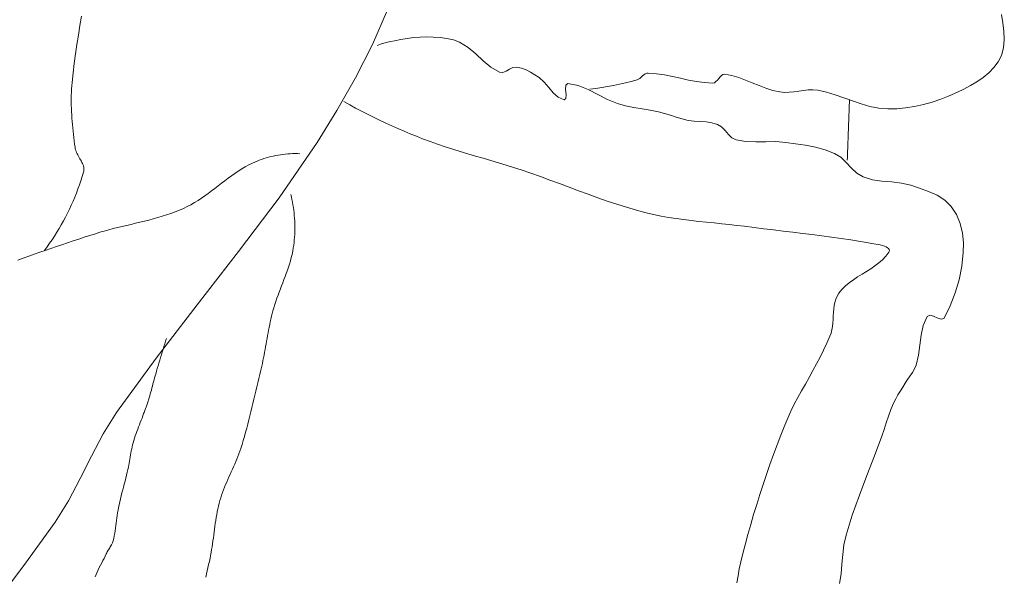
# Model space of a CAD drawing. Units: inches. Extents: x -15 to 423, y -713 to 71.
# Tile 14 of 24: x 333 to 362, y -324 to -308. Entities that reach past the tile are written whole.
import ezdxf

# ---------------------------------------------------------------- set-up
doc = ezdxf.new("R2010")
doc.units = ezdxf.units.IN
doc.header["$MEASUREMENT"] = 0
doc.layers.add('A-FURN', color=9, linetype='Continuous', lineweight=13)

# ---------------------------------------------------------------- blocks, each defined once
blk = doc.blocks.new('BED-DOUBLE')
for p, q in [((81.158, 34.884), (80.717, 33.859)), ((72.054, 34.699), (72.006, 34.418)), ((99.427, 34.751), (99.468, 34.498)), ((72.006, 34.418), (71.96, 34.136)), ((99.468, 34.498), (99.501, 34.248)), ((71.96, 34.136), (71.916, 33.855)), ((81.553, 34.002), (81.363, 33.968)), ((81.743, 34.034), (81.553, 34.002)), ((81.934, 34.06), (81.743, 34.034)), ((82.126, 34.077), (81.934, 34.06)), ((82.318, 34.081), (82.126, 34.077)), ((82.52, 34.075), (82.318, 34.081)), ((82.723, 34.063), (82.52, 34.075)), ((82.924, 34.037), (82.723, 34.063)), ((83.119, 33.992), (82.924, 34.037)), ((83.305, 33.921), (83.119, 33.992)), ((99.514, 34.001), (99.494, 33.761)), ((99.501, 34.248), (99.514, 34.001)), ((71.916, 33.855), (71.875, 33.573)), ((80.717, 33.859), (80.211, 32.862)), ((80.953, 33.862), (80.854, 33.825)), ((81.054, 33.894), (80.953, 33.862)), ((81.156, 33.923), (81.054, 33.894)), ((81.259, 33.948), (81.156, 33.923)), ((81.363, 33.968), (81.259, 33.948)), ((83.556, 33.766), (83.305, 33.921)), ((83.784, 33.574), (83.556, 33.766)), ((99.494, 33.761), (99.427, 33.528)), ((71.875, 33.573), (71.837, 33.29)), ((84.005, 33.372), (83.784, 33.574)), ((99.427, 33.528), (99.329, 33.34)), ((71.837, 33.29), (71.802, 33.008)), ((84.235, 33.184), (84.005, 33.372)), ((84.489, 33.037), (84.235, 33.184)), ((84.79, 33.12), (84.687, 33.064)), ((84.893, 33.168), (84.79, 33.12)), ((84.998, 33.18), (84.893, 33.168)), ((85.142, 33.148), (84.998, 33.18)), ((85.281, 33.097), (85.142, 33.148)), ((99.203, 33.169), (99.053, 33.014)), ((99.329, 33.34), (99.203, 33.169)), ((71.802, 33.008), (71.771, 32.725)), ((80.211, 32.862), (79.655, 31.89)), ((84.587, 33.027), (84.489, 33.037)), ((84.687, 33.064), (84.587, 33.027)), ((85.416, 33.031), (85.281, 33.097)), ((85.546, 32.954), (85.416, 33.031)), ((85.67, 32.872), (85.546, 32.954)), ((85.821, 32.738), (85.67, 32.872)), ((88.629, 32.82), (88.584, 32.801)), ((88.671, 32.849), (88.629, 32.82)), ((88.711, 32.883), (88.671, 32.849)), ((88.75, 32.919), (88.711, 32.883)), ((88.789, 32.953), (88.75, 32.919)), ((88.829, 32.982), (88.789, 32.953)), ((88.872, 33.001), (88.829, 32.982)), ((88.919, 33.007), (88.872, 33.001)), ((89.161, 32.986), (88.919, 33.007)), ((89.4, 32.95), (89.161, 32.986)), ((89.639, 32.903), (89.4, 32.95)), ((89.877, 32.851), (89.639, 32.903)), ((90.116, 32.799), (89.877, 32.851)), ((91.015, 32.845), (90.975, 32.795)), ((91.054, 32.895), (91.015, 32.845)), ((91.096, 32.937), (91.054, 32.895)), ((91.141, 32.965), (91.096, 32.937)), ((91.192, 32.971), (91.141, 32.965)), ((91.403, 32.931), (91.192, 32.971)), ((91.609, 32.871), (91.403, 32.931)), ((91.812, 32.797), (91.609, 32.871)), ((98.884, 32.874), (98.701, 32.747)), ((99.053, 33.014), (98.884, 32.874)), ((71.755, 32.532), (71.75, 32.436)), ((71.762, 32.629), (71.755, 32.532)), ((71.771, 32.725), (71.762, 32.629)), ((85.956, 32.578), (85.821, 32.738)), ((86.09, 32.42), (85.956, 32.578)), ((86.462, 32.647), (86.458, 32.521)), ((86.521, 32.696), (86.462, 32.647)), ((86.831, 32.634), (86.521, 32.696)), ((87.126, 32.514), (86.831, 32.634)), ((87.356, 32.547), (87.178, 32.524)), ((87.533, 32.573), (87.356, 32.547)), ((87.71, 32.603), (87.533, 32.573)), ((87.886, 32.636), (87.71, 32.603)), ((88.062, 32.672), (87.886, 32.636)), ((88.237, 32.712), (88.062, 32.672)), ((88.411, 32.755), (88.237, 32.712)), ((88.584, 32.801), (88.411, 32.755)), ((90.355, 32.755), (90.116, 32.799)), ((90.595, 32.722), (90.355, 32.755)), ((90.836, 32.707), (90.595, 32.722)), ((90.888, 32.719), (90.836, 32.707)), ((90.933, 32.75), (90.888, 32.719)), ((90.975, 32.795), (90.933, 32.75)), ((92.013, 32.716), (91.812, 32.797)), ((92.214, 32.634), (92.013, 32.716)), ((92.417, 32.558), (92.214, 32.634)), ((92.622, 32.492), (92.417, 32.558)), ((98.313, 32.528), (98.117, 32.433)), ((98.509, 32.632), (98.313, 32.528)), ((98.701, 32.747), (98.509, 32.632)), ((71.747, 32.34), (71.746, 32.243)), ((71.746, 32.243), (71.746, 32.147)), ((71.75, 32.436), (71.747, 32.34)), ((86.237, 32.289), (86.09, 32.42)), ((86.412, 32.213), (86.237, 32.289)), ((86.47, 32.251), (86.412, 32.213)), ((86.458, 32.521), (86.473, 32.372)), ((86.473, 32.372), (86.47, 32.251)), ((87.415, 32.365), (87.126, 32.514)), ((87.705, 32.216), (87.415, 32.365)), ((92.831, 32.445), (92.622, 32.492)), ((92.971, 32.431), (92.831, 32.445)), ((93.112, 32.434), (92.971, 32.431)), ((93.253, 32.448), (93.112, 32.434)), ((93.395, 32.468), (93.253, 32.448)), ((93.537, 32.488), (93.395, 32.468)), ((93.679, 32.503), (93.537, 32.488)), ((93.82, 32.507), (93.679, 32.503)), ((93.96, 32.495), (93.82, 32.507)), ((94.224, 32.44), (93.96, 32.495)), ((94.484, 32.363), (94.224, 32.44)), ((94.742, 32.273), (94.484, 32.363)), ((94.999, 32.179), (94.742, 32.273)), ((97.873, 32.324), (97.622, 32.227)), ((98.117, 32.433), (97.873, 32.324)), ((71.746, 32.147), (71.748, 32.05)), ((71.748, 32.05), (71.751, 31.954)), ((71.751, 31.954), (71.755, 31.857)), ((80.036, 32.061), (79.861, 32.158)), ((80.211, 31.966), (80.036, 32.061)), ((80.387, 31.873), (80.211, 31.966)), ((88.003, 32.096), (87.705, 32.216)), ((88.243, 32.032), (88.003, 32.096)), ((88.487, 31.984), (88.243, 32.032)), ((88.732, 31.944), (88.487, 31.984)), ((88.978, 31.903), (88.732, 31.944)), ((94.893, 31.858), (94.896, 31.949)), ((94.896, 31.949), (94.899, 32.039)), ((94.899, 32.039), (94.902, 32.129)), ((94.902, 32.129), (94.905, 32.22)), ((95.257, 32.09), (94.999, 32.179)), ((95.516, 32.015), (95.257, 32.09)), ((95.778, 31.962), (95.516, 32.015)), ((96.045, 31.939), (95.778, 31.962)), ((96.312, 31.945), (96.045, 31.939)), ((96.578, 31.969), (96.312, 31.945)), ((96.843, 32.011), (96.578, 31.969)), ((97.107, 32.069), (96.843, 32.011)), ((97.367, 32.141), (97.107, 32.069)), ((97.622, 32.227), (97.367, 32.141)), ((71.755, 31.857), (71.76, 31.761)), ((71.76, 31.761), (71.767, 31.664)), ((71.767, 31.664), (71.775, 31.568)), ((79.655, 31.89), (79.064, 30.944)), ((80.565, 31.782), (80.387, 31.873)), ((80.743, 31.692), (80.565, 31.782)), ((80.923, 31.605), (80.743, 31.692)), ((89.222, 31.853), (88.978, 31.903)), ((89.4, 31.805), (89.222, 31.853)), ((89.577, 31.751), (89.4, 31.805)), ((89.753, 31.695), (89.577, 31.751)), ((89.93, 31.642), (89.753, 31.695)), ((94.883, 31.587), (94.886, 31.678)), ((94.886, 31.678), (94.89, 31.768)), ((94.89, 31.768), (94.893, 31.858)), ((71.775, 31.568), (71.783, 31.471)), ((71.783, 31.471), (71.792, 31.375)), ((71.792, 31.375), (71.802, 31.278)), ((81.104, 31.52), (80.923, 31.605)), ((81.285, 31.437), (81.104, 31.52)), ((81.468, 31.355), (81.285, 31.437)), ((81.651, 31.276), (81.468, 31.355)), ((90.109, 31.598), (89.93, 31.642)), ((90.284, 31.573), (90.109, 31.598)), ((90.462, 31.562), (90.284, 31.573)), ((90.639, 31.551), (90.462, 31.562)), ((90.814, 31.528), (90.639, 31.551)), ((90.981, 31.479), (90.814, 31.528)), ((91.101, 31.403), (90.981, 31.479)), ((91.205, 31.296), (91.101, 31.403)), ((94.874, 31.317), (94.877, 31.407)), ((94.877, 31.407), (94.88, 31.497)), ((94.88, 31.497), (94.883, 31.587)), ((71.802, 31.278), (71.813, 31.182)), ((71.813, 31.182), (71.824, 31.086)), ((71.824, 31.086), (71.836, 30.99)), ((81.835, 31.199), (81.651, 31.276)), ((82.02, 31.124), (81.835, 31.199)), ((82.205, 31.052), (82.02, 31.124)), ((91.303, 31.181), (91.205, 31.296)), ((91.408, 31.082), (91.303, 31.181)), ((91.533, 31.019), (91.408, 31.082)), ((94.864, 31.046), (94.867, 31.136)), ((94.867, 31.136), (94.871, 31.226)), ((94.871, 31.226), (94.874, 31.317)), ((71.836, 30.99), (71.848, 30.894)), ((71.848, 30.894), (71.86, 30.798)), ((71.86, 30.798), (71.867, 30.759)), ((79.064, 30.944), (77.93, 29.295)), ((82.427, 30.969), (82.205, 31.052)), ((82.65, 30.89), (82.427, 30.969)), ((82.874, 30.815), (82.65, 30.89)), ((83.099, 30.743), (82.874, 30.815)), ((91.823, 30.969), (91.533, 31.019)), ((92.118, 30.958), (91.823, 30.969)), ((92.416, 30.963), (92.118, 30.958)), ((92.714, 30.966), (92.416, 30.963)), ((93.009, 30.944), (92.714, 30.966)), ((93.304, 30.904), (93.009, 30.944)), ((93.601, 30.858), (93.304, 30.904)), ((93.894, 30.8), (93.601, 30.858)), ((94.181, 30.722), (93.894, 30.8)), ((94.852, 30.684), (94.855, 30.775)), ((94.855, 30.775), (94.858, 30.865)), ((94.858, 30.865), (94.861, 30.955)), ((94.861, 30.955), (94.864, 31.046)), ((71.867, 30.759), (71.877, 30.721)), ((71.877, 30.721), (71.891, 30.683)), ((71.891, 30.683), (71.906, 30.645)), ((71.906, 30.645), (71.924, 30.608)), ((71.924, 30.608), (71.944, 30.57)), ((71.944, 30.57), (71.964, 30.533)), ((71.964, 30.533), (71.985, 30.496)), ((71.985, 30.496), (72.007, 30.459)), ((77.48, 30.462), (77.549, 30.483)), ((77.549, 30.483), (77.619, 30.503)), ((77.619, 30.503), (77.689, 30.522)), ((77.689, 30.522), (77.76, 30.538)), ((77.76, 30.538), (77.831, 30.553)), ((77.831, 30.553), (77.902, 30.566)), ((77.902, 30.566), (77.974, 30.578)), ((77.974, 30.578), (78.046, 30.588)), ((78.046, 30.588), (78.118, 30.595)), ((78.118, 30.595), (78.19, 30.602)), ((78.19, 30.602), (78.263, 30.606)), ((78.263, 30.606), (78.335, 30.609)), ((78.335, 30.609), (78.407, 30.61)), ((78.407, 30.61), (78.479, 30.609)), ((78.479, 30.609), (78.551, 30.606)), ((83.325, 30.673), (83.099, 30.743)), ((83.552, 30.605), (83.325, 30.673)), ((83.779, 30.538), (83.552, 30.605)), ((84.006, 30.471), (83.779, 30.538)), ((94.458, 30.617), (94.181, 30.722)), ((94.644, 30.5), (94.458, 30.617)), ((94.808, 30.347), (94.644, 30.5)), ((94.842, 30.414), (94.845, 30.504)), ((94.845, 30.504), (94.848, 30.594)), ((94.848, 30.594), (94.852, 30.684)), ((72.007, 30.459), (72.027, 30.423)), ((72.027, 30.423), (72.048, 30.386)), ((72.048, 30.386), (72.066, 30.349)), ((72.066, 30.349), (72.083, 30.313)), ((72.083, 30.313), (72.098, 30.276)), ((72.098, 30.276), (72.11, 30.239)), ((72.11, 30.239), (72.119, 30.203)), ((72.119, 30.203), (72.125, 30.166)), ((76.822, 30.154), (76.927, 30.216)), ((76.927, 30.216), (77.035, 30.275)), ((77.035, 30.275), (77.145, 30.33)), ((77.145, 30.33), (77.21, 30.359)), ((77.21, 30.359), (77.276, 30.387)), ((77.276, 30.387), (77.343, 30.414)), ((77.343, 30.414), (77.411, 30.439)), ((77.411, 30.439), (77.48, 30.462)), ((84.233, 30.404), (84.006, 30.471)), ((84.46, 30.337), (84.233, 30.404)), ((84.686, 30.269), (84.46, 30.337)), ((84.912, 30.198), (84.686, 30.269)), ((85.137, 30.125), (84.912, 30.198)), ((94.964, 30.181), (94.808, 30.347)), ((95.128, 30.029), (94.964, 30.181)), ((72.076, 29.929), (72.035, 29.805)), ((72.114, 30.054), (72.076, 29.929)), ((72.122, 30.091), (72.114, 30.054)), ((72.126, 30.129), (72.122, 30.091)), ((72.125, 30.166), (72.126, 30.129)), ((76.415, 29.875), (76.515, 29.948)), ((76.515, 29.948), (76.616, 30.019)), ((76.616, 30.019), (76.718, 30.088)), ((76.718, 30.088), (76.822, 30.154)), ((85.424, 30.028), (85.137, 30.125)), ((85.709, 29.927), (85.424, 30.028)), ((85.993, 29.823), (85.709, 29.927)), ((95.316, 29.916), (95.128, 30.029)), ((95.589, 29.834), (95.316, 29.916)), ((71.993, 29.682), (71.948, 29.56)), ((72.035, 29.805), (71.993, 29.682)), ((76.021, 29.575), (76.12, 29.65)), ((76.12, 29.65), (76.218, 29.726)), ((76.218, 29.726), (76.316, 29.801)), ((76.316, 29.801), (76.415, 29.875)), ((86.277, 29.718), (85.993, 29.823)), ((86.561, 29.612), (86.277, 29.718)), ((86.845, 29.506), (86.561, 29.612)), ((95.873, 29.793), (95.589, 29.834)), ((96.162, 29.768), (95.873, 29.793)), ((96.45, 29.735), (96.162, 29.768)), ((96.728, 29.668), (96.45, 29.735)), ((96.993, 29.581), (96.728, 29.668)), ((71.852, 29.317), (71.8, 29.196)), ((71.901, 29.438), (71.852, 29.317)), ((71.948, 29.56), (71.901, 29.438)), ((75.622, 29.284), (75.724, 29.354)), ((75.724, 29.354), (75.824, 29.426)), ((75.824, 29.426), (75.923, 29.5)), ((75.923, 29.5), (76.021, 29.575)), ((78.278, 29.398), (78.297, 29.321)), ((78.297, 29.321), (78.315, 29.242)), ((87.129, 29.401), (86.845, 29.506)), ((87.414, 29.298), (87.129, 29.401)), ((97.26, 29.486), (96.993, 29.581)), ((97.515, 29.372), (97.26, 29.486)), ((97.746, 29.225), (97.515, 29.372)), ((71.747, 29.077), (71.691, 28.958)), ((71.8, 29.196), (71.747, 29.077)), ((75.09, 28.98), (75.201, 29.033)), ((75.201, 29.033), (75.31, 29.09)), ((75.31, 29.09), (75.416, 29.151)), ((75.416, 29.151), (75.52, 29.216)), ((75.52, 29.216), (75.622, 29.284)), ((77.93, 29.295), (76.727, 27.695)), ((78.315, 29.242), (78.33, 29.164)), ((78.33, 29.164), (78.345, 29.085)), ((78.345, 29.085), (78.357, 29.005)), ((87.699, 29.198), (87.414, 29.298)), ((87.986, 29.102), (87.699, 29.198)), ((88.275, 29.012), (87.986, 29.102)), ((88.565, 28.927), (88.275, 29.012)), ((97.937, 29.036), (97.746, 29.225)), ((98.089, 28.796), (97.937, 29.036)), ((71.574, 28.724), (71.512, 28.609)), ((71.634, 28.841), (71.574, 28.724)), ((71.691, 28.958), (71.634, 28.841)), ((74.322, 28.706), (74.452, 28.745)), ((74.452, 28.745), (74.582, 28.786)), ((74.582, 28.786), (74.711, 28.829)), ((74.711, 28.829), (74.839, 28.876)), ((74.839, 28.876), (74.965, 28.926)), ((74.965, 28.926), (75.09, 28.98)), ((78.357, 29.005), (78.368, 28.925)), ((78.368, 28.925), (78.378, 28.845)), ((78.378, 28.845), (78.386, 28.765)), ((78.386, 28.765), (78.392, 28.685)), ((88.857, 28.849), (88.565, 28.927)), ((89.078, 28.797), (88.857, 28.849)), ((89.3, 28.752), (89.078, 28.797)), ((89.523, 28.712), (89.3, 28.752)), ((98.197, 28.529), (98.089, 28.796)), ((71.448, 28.495), (71.383, 28.381)), ((71.512, 28.609), (71.448, 28.495)), ((73.126, 28.411), (73.259, 28.443)), ((73.259, 28.443), (73.392, 28.475)), ((73.392, 28.475), (73.526, 28.506)), ((73.526, 28.506), (73.659, 28.538)), ((73.659, 28.538), (73.793, 28.569)), ((73.793, 28.569), (73.926, 28.602)), ((73.926, 28.602), (74.058, 28.635)), ((74.058, 28.635), (74.19, 28.67)), ((74.19, 28.67), (74.322, 28.706)), ((78.392, 28.685), (78.397, 28.604)), ((78.397, 28.604), (78.4, 28.524)), ((78.4, 28.524), (78.401, 28.443)), ((78.401, 28.443), (78.401, 28.362)), ((89.748, 28.678), (89.523, 28.712)), ((89.973, 28.647), (89.748, 28.678)), ((90.198, 28.62), (89.973, 28.647)), ((90.425, 28.595), (90.198, 28.62)), ((90.651, 28.572), (90.425, 28.595)), ((90.878, 28.549), (90.651, 28.572)), ((91.104, 28.526), (90.878, 28.549)), ((91.33, 28.502), (91.104, 28.526)), ((91.556, 28.476), (91.33, 28.502)), ((91.782, 28.447), (91.556, 28.476)), ((92.069, 28.41), (91.782, 28.447)), ((98.265, 28.245), (98.197, 28.529)), ((71.246, 28.159), (71.175, 28.05)), ((71.315, 28.27), (71.246, 28.159)), ((71.383, 28.381), (71.315, 28.27)), ((72.136, 28.12), (72.302, 28.174)), ((72.302, 28.174), (72.468, 28.228)), ((72.468, 28.228), (72.598, 28.269)), ((72.598, 28.269), (72.729, 28.307)), ((72.729, 28.307), (72.861, 28.343)), ((72.861, 28.343), (72.993, 28.378)), ((72.993, 28.378), (73.126, 28.411)), ((78.396, 28.201), (78.392, 28.121)), ((78.4, 28.282), (78.396, 28.201)), ((78.401, 28.362), (78.4, 28.282)), ((92.357, 28.373), (92.069, 28.41)), ((92.645, 28.338), (92.357, 28.373)), ((92.934, 28.304), (92.645, 28.338)), ((93.222, 28.269), (92.934, 28.304)), ((93.51, 28.235), (93.222, 28.269)), ((93.798, 28.2), (93.51, 28.235)), ((94.086, 28.163), (93.798, 28.2)), ((94.374, 28.125), (94.086, 28.163)), ((98.296, 27.954), (98.265, 28.245)), ((71.101, 27.942), (71.026, 27.835)), ((71.175, 28.05), (71.101, 27.942)), ((71.141, 27.788), (71.307, 27.845)), ((71.307, 27.845), (71.472, 27.9)), ((71.472, 27.9), (71.638, 27.956)), ((71.638, 27.956), (71.804, 28.011)), ((71.804, 28.011), (71.97, 28.065)), ((71.97, 28.065), (72.136, 28.12)), ((78.367, 27.882), (78.356, 27.803)), ((78.377, 27.961), (78.367, 27.882)), ((78.385, 28.041), (78.377, 27.961)), ((78.392, 28.121), (78.385, 28.041)), ((94.661, 28.085), (94.374, 28.125)), ((94.948, 28.043), (94.661, 28.085)), ((95.235, 27.997), (94.948, 28.043)), ((95.52, 27.948), (95.235, 27.997)), ((95.572, 27.94), (95.52, 27.948)), ((95.63, 27.93), (95.572, 27.94)), ((95.692, 27.919), (95.63, 27.93)), ((95.757, 27.907), (95.692, 27.919)), ((95.823, 27.892), (95.757, 27.907)), ((95.886, 27.876), (95.823, 27.892)), ((95.945, 27.858), (95.886, 27.876)), ((95.997, 27.836), (95.945, 27.858)), ((96.04, 27.812), (95.997, 27.836)), ((98.293, 27.667), (98.296, 27.954)), ((70.317, 27.499), (70.481, 27.558)), ((70.481, 27.558), (70.646, 27.616)), ((70.646, 27.616), (70.811, 27.674)), ((70.811, 27.674), (70.976, 27.732)), ((71.026, 27.835), (70.95, 27.73)), ((70.976, 27.732), (71.141, 27.788)), ((76.727, 27.695), (75.494, 26.115)), ((78.319, 27.61), (78.296, 27.515)), ((78.339, 27.706), (78.319, 27.61)), ((78.356, 27.803), (78.339, 27.706)), ((95.893, 27.455), (95.992, 27.563)), ((95.992, 27.563), (96.078, 27.682)), ((96.072, 27.785), (96.04, 27.812)), ((96.09, 27.755), (96.072, 27.785)), ((96.078, 27.682), (96.093, 27.72)), ((96.093, 27.72), (96.09, 27.755)), ((98.248, 27.261), (98.293, 27.667)), ((70.153, 27.439), (70.317, 27.499)), ((78.243, 27.326), (78.213, 27.233)), ((78.271, 27.42), (78.243, 27.326)), ((78.296, 27.515), (78.271, 27.42)), ((95.539, 27.183), (95.664, 27.267)), ((95.664, 27.267), (95.783, 27.357)), ((95.783, 27.357), (95.893, 27.455)), ((98.169, 26.859), (98.248, 27.261)), ((78.147, 27.047), (78.113, 26.954)), ((78.181, 27.139), (78.147, 27.047)), ((78.213, 27.233), (78.181, 27.139)), ((95.149, 26.941), (95.279, 27.022)), ((95.279, 27.022), (95.41, 27.101)), ((95.41, 27.101), (95.539, 27.183)), ((78.006, 26.678), (77.97, 26.585)), ((78.042, 26.77), (78.006, 26.678)), ((78.078, 26.862), (78.042, 26.77)), ((78.113, 26.954), (78.078, 26.862)), ((94.682, 26.57), (94.786, 26.674)), ((94.786, 26.674), (94.9, 26.77)), ((94.9, 26.77), (95.022, 26.858)), ((95.022, 26.858), (95.149, 26.941)), ((98.054, 26.464), (98.169, 26.859)), ((77.9, 26.401), (77.866, 26.308)), ((77.934, 26.493), (77.9, 26.401)), ((77.97, 26.585), (77.934, 26.493)), ((94.539, 26.37), (94.59, 26.455)), ((94.59, 26.455), (94.682, 26.57)), ((97.904, 26.082), (98.054, 26.464)), ((75.494, 26.115), (74.271, 24.528)), ((77.802, 26.121), (77.774, 26.027)), ((77.833, 26.215), (77.802, 26.121)), ((77.866, 26.308), (77.833, 26.215)), ((94.439, 25.988), (94.453, 26.088)), ((94.453, 26.088), (94.473, 26.186)), ((94.473, 26.186), (94.501, 26.28)), ((94.501, 26.28), (94.539, 26.37)), ((97.721, 25.718), (97.904, 26.082)), ((77.726, 25.851), (77.706, 25.77)), ((77.747, 25.932), (77.726, 25.851)), ((77.774, 26.027), (77.747, 25.932)), ((94.423, 25.782), (94.43, 25.886)), ((94.43, 25.886), (94.439, 25.988)), ((97.217, 25.769), (97.294, 25.805)), ((97.294, 25.805), (97.407, 25.772)), ((77.652, 25.524), (77.636, 25.442)), ((77.669, 25.606), (77.652, 25.524)), ((77.687, 25.688), (77.669, 25.606)), ((77.706, 25.77), (77.687, 25.688)), ((94.399, 25.472), (94.41, 25.575)), ((94.41, 25.575), (94.417, 25.678)), ((94.417, 25.678), (94.423, 25.782)), ((97.037, 25.21), (97.1, 25.5)), ((97.1, 25.5), (97.217, 25.769)), ((97.407, 25.772), (97.532, 25.714)), ((97.532, 25.714), (97.645, 25.681)), ((97.645, 25.681), (97.721, 25.718)), ((77.604, 25.277), (77.589, 25.195)), ((77.62, 25.36), (77.604, 25.277)), ((77.636, 25.442), (77.62, 25.36)), ((94.326, 25.179), (94.359, 25.273)), ((94.359, 25.273), (94.382, 25.372)), ((94.382, 25.372), (94.399, 25.472)), ((96.999, 24.911), (97.037, 25.21)), ((74.528, 24.953), (74.504, 24.871)), ((74.553, 25.034), (74.528, 24.953)), ((74.579, 25.115), (74.553, 25.034)), ((77.545, 24.947), (77.53, 24.864)), ((77.56, 25.029), (77.545, 24.947)), ((77.574, 25.112), (77.56, 25.029)), ((77.589, 25.195), (77.574, 25.112)), ((94.138, 24.762), (94.235, 24.969)), ((94.235, 24.969), (94.326, 25.179)), ((96.959, 24.61), (96.999, 24.911)), ((74.43, 24.626), (74.405, 24.545)), ((74.454, 24.708), (74.43, 24.626)), ((74.479, 24.79), (74.454, 24.708)), ((74.504, 24.871), (74.479, 24.79)), ((77.485, 24.617), (77.468, 24.534)), ((77.5, 24.699), (77.485, 24.617)), ((77.516, 24.782), (77.5, 24.699)), ((77.53, 24.864), (77.516, 24.782)), ((94.035, 24.558), (94.138, 24.762)), ((74.271, 24.528), (73.096, 22.907)), ((74.357, 24.381), (74.333, 24.3)), ((74.381, 24.463), (74.357, 24.381)), ((74.405, 24.545), (74.381, 24.463)), ((77.434, 24.37), (77.415, 24.288)), ((77.452, 24.452), (77.434, 24.37)), ((77.468, 24.534), (77.452, 24.452)), ((93.818, 24.155), (93.928, 24.356)), ((93.928, 24.356), (94.035, 24.558)), ((96.841, 24.205), (96.89, 24.32)), ((96.89, 24.32), (96.959, 24.61)), ((74.261, 24.054), (74.244, 23.995)), ((74.285, 24.136), (74.261, 24.054)), ((74.309, 24.218), (74.285, 24.136)), ((74.333, 24.3), (74.309, 24.218)), ((77.358, 24.042), (77.33, 23.918)), ((77.387, 24.165), (77.358, 24.042)), ((77.415, 24.288), (77.387, 24.165)), ((93.706, 23.955), (93.818, 24.155)), ((96.707, 23.993), (96.778, 24.097)), ((96.778, 24.097), (96.841, 24.205)), ((74.18, 23.757), (74.164, 23.697)), ((74.196, 23.817), (74.18, 23.757)), ((74.212, 23.876), (74.196, 23.817)), ((74.228, 23.936), (74.212, 23.876)), ((74.244, 23.995), (74.228, 23.936)), ((77.301, 23.795), (77.272, 23.672)), ((77.33, 23.918), (77.301, 23.795)), ((93.482, 23.555), (93.593, 23.755)), ((93.593, 23.755), (93.706, 23.955)), ((96.494, 23.666), (96.566, 23.783)), ((96.566, 23.783), (96.634, 23.889)), ((96.634, 23.889), (96.707, 23.993)), ((74.1, 23.46), (74.083, 23.4)), ((74.116, 23.519), (74.1, 23.46)), ((74.132, 23.578), (74.116, 23.519)), ((74.148, 23.638), (74.132, 23.578)), ((74.164, 23.697), (74.148, 23.638)), ((77.244, 23.548), (77.215, 23.425)), ((77.272, 23.672), (77.244, 23.548)), ((93.372, 23.354), (93.482, 23.555)), ((96.349, 23.432), (96.421, 23.549)), ((96.421, 23.549), (96.494, 23.666)), ((74.006, 23.157), (73.995, 23.125)), ((74.017, 23.188), (74.006, 23.157)), ((74.028, 23.219), (74.017, 23.188)), ((74.038, 23.25), (74.028, 23.219)), ((74.048, 23.282), (74.038, 23.25)), ((74.066, 23.341), (74.048, 23.282)), ((74.083, 23.4), (74.066, 23.341)), ((77.156, 23.179), (77.126, 23.056)), ((77.185, 23.302), (77.156, 23.179)), ((77.215, 23.425), (77.185, 23.302)), ((93.164, 22.947), (93.265, 23.152)), ((93.265, 23.152), (93.372, 23.354)), ((96.141, 22.996), (96.221, 23.189)), ((96.221, 23.189), (96.281, 23.312)), ((96.281, 23.312), (96.349, 23.432)), ((73.096, 22.907), (72.702, 22.273)), ((73.902, 22.877), (73.878, 22.811)), ((73.913, 22.909), (73.902, 22.877)), ((73.925, 22.94), (73.913, 22.909)), ((73.937, 22.971), (73.925, 22.94)), ((73.948, 23.002), (73.937, 22.971)), ((73.96, 23.032), (73.948, 23.002)), ((73.972, 23.063), (73.96, 23.032)), ((73.983, 23.094), (73.972, 23.063)), ((73.995, 23.125), (73.983, 23.094)), ((77.096, 22.933), (77.065, 22.81)), ((77.126, 23.056), (77.096, 22.933)), ((93.068, 22.74), (93.164, 22.947)), ((96.069, 22.8), (96.141, 22.996)), ((73.802, 22.612), (73.776, 22.546)), ((73.827, 22.678), (73.802, 22.612)), ((73.853, 22.744), (73.827, 22.678)), ((73.878, 22.811), (73.853, 22.744)), ((77.001, 22.565), (76.968, 22.443)), ((77.033, 22.688), (77.001, 22.565)), ((77.065, 22.81), (77.033, 22.688)), ((92.979, 22.53), (93.068, 22.74)), ((95.935, 22.404), (96.002, 22.602)), ((96.002, 22.602), (96.069, 22.8)), ((72.702, 22.273), (72.35, 21.612)), ((73.676, 22.28), (73.653, 22.213)), ((73.701, 22.347), (73.676, 22.28)), ((73.725, 22.413), (73.701, 22.347)), ((73.751, 22.48), (73.725, 22.413)), ((73.776, 22.546), (73.751, 22.48)), ((76.935, 22.321), (76.9, 22.199)), ((76.968, 22.443), (76.935, 22.321)), ((92.864, 22.239), (92.979, 22.53)), ((95.867, 22.207), (95.935, 22.404)), ((73.59, 22.01), (73.573, 21.95)), ((73.609, 22.079), (73.59, 22.01)), ((73.631, 22.146), (73.609, 22.079)), ((73.653, 22.213), (73.631, 22.146)), ((76.865, 22.078), (76.829, 21.956)), ((76.9, 22.199), (76.865, 22.078)), ((92.753, 21.948), (92.864, 22.239)), ((95.648, 21.619), (95.867, 22.207)), ((73.522, 21.707), (73.512, 21.646)), ((73.534, 21.768), (73.522, 21.707)), ((73.546, 21.829), (73.534, 21.768)), ((73.559, 21.89), (73.546, 21.829)), ((73.573, 21.95), (73.559, 21.89)), ((76.766, 21.756), (76.739, 21.678)), ((76.792, 21.835), (76.766, 21.756)), ((76.829, 21.956), (76.792, 21.835)), ((92.644, 21.655), (92.753, 21.948)), ((72.35, 21.612), (72.012, 20.943)), ((73.47, 21.4), (73.459, 21.339)), ((73.481, 21.462), (73.47, 21.4)), ((73.491, 21.523), (73.481, 21.462)), ((73.501, 21.585), (73.491, 21.523)), ((73.512, 21.646), (73.501, 21.585)), ((76.647, 21.447), (76.614, 21.371)), ((76.679, 21.524), (76.647, 21.447)), ((76.709, 21.601), (76.679, 21.524)), ((76.739, 21.678), (76.709, 21.601)), ((92.539, 21.361), (92.644, 21.655)), ((95.422, 21.034), (95.648, 21.619)), ((73.414, 21.13), (73.393, 21.042)), ((73.434, 21.217), (73.414, 21.13)), ((73.447, 21.278), (73.434, 21.217)), ((73.459, 21.339), (73.447, 21.278)), ((76.511, 21.143), (76.476, 21.067)), ((76.546, 21.219), (76.511, 21.143)), ((76.58, 21.294), (76.546, 21.219)), ((76.614, 21.371), (76.58, 21.294)), ((92.436, 21.066), (92.539, 21.361)), ((72.012, 20.943), (71.661, 20.282)), ((73.348, 20.867), (73.326, 20.779)), ((73.371, 20.954), (73.348, 20.867)), ((73.393, 21.042), (73.371, 20.954)), ((76.373, 20.84), (76.34, 20.763)), ((76.407, 20.916), (76.373, 20.84)), ((76.441, 20.991), (76.407, 20.916)), ((76.476, 21.067), (76.441, 20.991)), ((92.337, 20.77), (92.436, 21.066)), ((95.2, 20.447), (95.422, 21.034)), ((73.257, 20.517), (73.235, 20.429)), ((73.28, 20.604), (73.257, 20.517)), ((73.303, 20.692), (73.28, 20.604)), ((73.326, 20.779), (73.303, 20.692)), ((76.248, 20.532), (76.221, 20.454)), ((76.278, 20.61), (76.248, 20.532)), ((76.308, 20.687), (76.278, 20.61)), ((76.34, 20.763), (76.308, 20.687)), ((92.24, 20.473), (92.337, 20.77)), ((71.661, 20.282), (71.268, 19.647)), ((73.193, 20.254), (73.173, 20.166)), ((73.214, 20.342), (73.193, 20.254)), ((73.235, 20.429), (73.214, 20.342)), ((76.171, 20.296), (76.149, 20.211)), ((76.195, 20.375), (76.171, 20.296)), ((76.221, 20.454), (76.195, 20.375)), ((92.146, 20.175), (92.24, 20.473)), ((94.99, 19.857), (95.2, 20.447)), ((73.126, 19.926), (73.115, 19.85)), ((73.139, 20.002), (73.126, 19.926)), ((73.154, 20.078), (73.139, 20.002)), ((73.173, 20.166), (73.154, 20.078)), ((76.092, 19.956), (76.076, 19.87)), ((76.109, 20.041), (76.092, 19.956)), ((76.128, 20.127), (76.109, 20.041)), ((76.149, 20.211), (76.128, 20.127)), ((92.055, 19.876), (92.146, 20.175)), ((71.268, 19.647), (70.336, 18.355)), ((73.095, 19.697), (73.085, 19.621)), ((73.104, 19.774), (73.095, 19.697)), ((73.115, 19.85), (73.104, 19.774)), ((76.048, 19.698), (76.035, 19.611)), ((76.062, 19.784), (76.048, 19.698)), ((76.076, 19.87), (76.062, 19.784)), ((91.967, 19.576), (92.055, 19.876)), ((94.804, 19.259), (94.99, 19.857)), ((73.054, 19.392), (73.042, 19.316)), ((73.065, 19.468), (73.054, 19.392)), ((73.076, 19.544), (73.065, 19.468)), ((73.085, 19.621), (73.076, 19.544)), ((75.999, 19.351), (75.988, 19.264)), ((76.011, 19.438), (75.999, 19.351)), ((76.023, 19.524), (76.011, 19.438)), ((76.035, 19.611), (76.023, 19.524)), ((91.882, 19.276), (91.967, 19.576)), ((72.984, 19.059), (72.972, 19.028)), ((72.994, 19.09), (72.984, 19.059)), ((73.012, 19.165), (72.994, 19.09)), ((73.028, 19.24), (73.012, 19.165)), ((73.042, 19.316), (73.028, 19.24)), ((75.965, 19.09), (75.952, 19.004)), ((75.976, 19.177), (75.965, 19.09)), ((75.988, 19.264), (75.976, 19.177)), ((91.799, 18.975), (91.882, 19.276)), ((94.742, 18.977), (94.804, 19.259)), ((72.821, 18.766), (72.805, 18.737)), ((72.838, 18.795), (72.821, 18.766)), ((72.856, 18.824), (72.838, 18.795)), ((72.874, 18.852), (72.856, 18.824)), ((72.892, 18.881), (72.874, 18.852)), ((72.91, 18.91), (72.892, 18.881)), ((72.927, 18.938), (72.91, 18.91)), ((72.943, 18.968), (72.927, 18.938)), ((72.958, 18.997), (72.943, 18.968)), ((72.972, 19.028), (72.958, 18.997)), ((75.925, 18.831), (75.911, 18.745)), ((75.939, 18.917), (75.925, 18.831)), ((75.952, 19.004), (75.939, 18.917)), ((91.719, 18.673), (91.799, 18.975)), ((94.707, 18.69), (94.742, 18.977)), ((72.688, 18.502), (72.653, 18.434)), ((72.723, 18.57), (72.688, 18.502)), ((72.757, 18.638), (72.723, 18.57)), ((72.79, 18.707), (72.757, 18.638)), ((72.805, 18.737), (72.79, 18.707)), ((75.857, 18.48), (75.836, 18.386)), ((75.877, 18.573), (75.857, 18.48)), ((75.894, 18.659), (75.877, 18.573)), ((75.911, 18.745), (75.894, 18.659)), ((91.627, 18.261), (91.669, 18.468)), ((91.669, 18.468), (91.719, 18.673)), ((94.683, 18.401), (94.707, 18.69)), ((70.336, 18.355), (69.362, 17.092)), ((72.55, 18.229), (72.518, 18.16)), ((72.583, 18.298), (72.55, 18.229)), ((72.618, 18.366), (72.583, 18.298)), ((72.653, 18.434), (72.618, 18.366)), ((75.793, 18.2), (75.772, 18.106)), ((75.815, 18.293), (75.793, 18.2)), ((75.836, 18.386), (75.815, 18.293)), ((91.59, 18.053), (91.627, 18.261)), ((94.657, 18.111), (94.683, 18.401)), ((72.488, 18.091), (72.461, 18.02)), ((72.518, 18.16), (72.488, 18.091)), ((75.772, 18.106), (75.749, 18.013)), ((91.558, 17.844), (91.59, 18.053)), ((94.613, 17.825), (94.657, 18.111))]:
    blk.add_line(p, q)

msp = doc.modelspace()

# ---------------------------------------------------------------- block references
at = {"layer": 'A-FURN'}
msp.add_blockref('BED-DOUBLE', (262.678, -342.175), dxfattribs=at)

doc.saveas('drawing.dxf')
